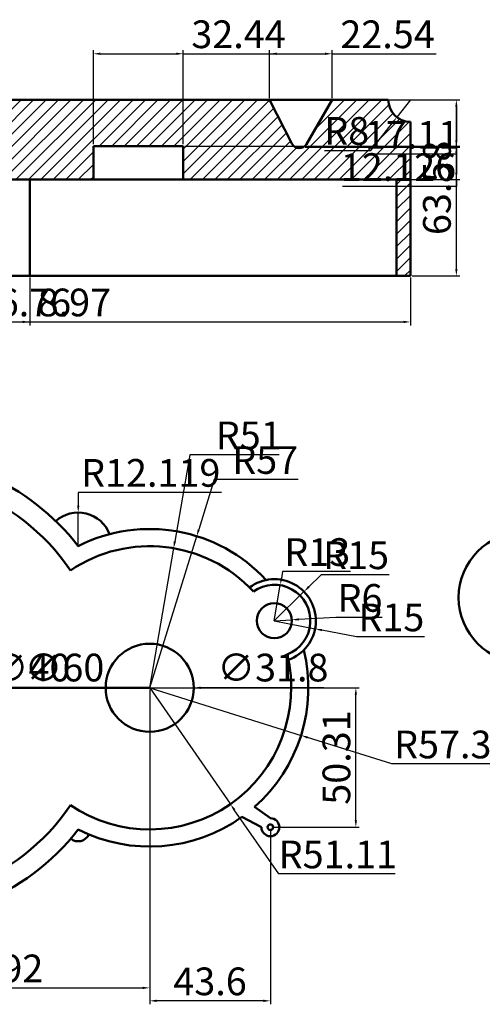
# Model space of a CAD drawing. Units: millimetres. Extents: x 828 to 2987, y 979 to 1807.
# Tile 2 of 6: x 1058 to 1225, y 1105 to 1460. Entities that reach past the tile are written whole.
import ezdxf

# ---------------------------------------------------------------- set-up
doc = ezdxf.new("R2010")
doc.units = ezdxf.units.MM
for name, color, linetype, lineweight in [('M-DIMS', 2, 'Continuous', 25), ('M-HATC', 8, 'Continuous', 18), ('M-OUTL', 7, 'Continuous', 50)]:
    doc.layers.add(name, color=color, linetype=linetype, lineweight=lineweight)
doc.styles.get("Standard").update_dxf_attribs({"font": 'arial.ttf'})
doc.dimstyles.new('ISO-25', dxfattribs={"dimtxt": 10, "dimasz": 2.5, "dimexe": 1.25, "dimexo": 0.625, "dimtad": 1, "dimtoh": 1, "dimdec": 0, "dimtxsty": 'Standard', "dimcen": 2.5, "dimadec": 0, "dimazin": 0, "dimtfac": 1, "dimtdec": 0, "dimtmove": 0, "dimatfit": 3, "dimfxl": 1, "dimarcsym": 0})

# ---------------------------------------------------------------- blocks, each defined once
blk = doc.blocks.new('*D17')
at = {"layer": 'Defpoints', "color": 0, "transparency": 16777216}
for p in [(1013.21, 1219.26), (1105.21, 1219.26), (1105.21, 1110.96)]:
    blk.add_point(p, dxfattribs=at)
at = {"layer": 'M-DIMS', "color": 0, "lineweight": -2, "transparency": 16777216}
for p, q in [((1013.21, 1218.63), (1013.21, 1109.71)), ((1105.21, 1218.63), (1105.21, 1109.71)), ((1015.71, 1110.96), (1102.71, 1110.96))]:
    blk.add_line(p, q, dxfattribs=at)
at = {"layer": 'M-DIMS', "color": 0, "transparency": 16777216}
for points in [[(1015.71, 1111.37), (1015.71, 1110.54), (1013.21, 1110.96)], [(1102.71, 1111.37), (1102.71, 1110.54), (1105.21, 1110.96)]]:
    blk.add_solid(points, dxfattribs=at)
at = {"layer": 'M-DIMS', "color": 0, "transparency": 16777216, "insert": (1059.21, 1116.69), "char_height": 10, "attachment_point": 5}
blk.add_mtext('92', dxfattribs=at)
blk = doc.blocks.new('*D20')
at = {"layer": 'Defpoints', "color": 0, "transparency": 16777216}
for p in [(1122.19, 1273.99), (1105.21, 1219.26)]:
    blk.add_point(p, dxfattribs=at)
at = {"layer": 'M-DIMS', "color": 0, "lineweight": -2, "transparency": 16777216}
for p, q in [((1128.54, 1294.46), (1122.93, 1276.38)), ((1158.89, 1294.46), (1128.54, 1294.46)), ((1105.21, 1219.26), (1122.19, 1273.99))]:
    blk.add_line(p, q, dxfattribs=at)
at = {"layer": 'M-DIMS', "color": 0, "transparency": 16777216}
blk.add_solid([(1122.54, 1276.5), (1123.33, 1276.25), (1122.19, 1273.99)], dxfattribs=at)
at = {"layer": 'M-DIMS', "color": 0, "transparency": 16777216, "insert": (1146.94, 1300.17), "char_height": 10, "attachment_point": 5}
blk.add_mtext('R57', dxfattribs=at)
blk = doc.blocks.new('*D21')
at = {"layer": 'Defpoints', "color": 0, "transparency": 16777216}
for p in [(1113.88, 1269.63), (1105.21, 1219.26)]:
    blk.add_point(p, dxfattribs=at)
at = {"layer": 'M-DIMS', "color": 0, "lineweight": -2, "transparency": 16777216}
for p, q in [((1119.67, 1303.32), (1114.3, 1272.1)), ((1151.97, 1303.32), (1119.67, 1303.32)), ((1105.21, 1219.26), (1113.88, 1269.63))]:
    blk.add_line(p, q, dxfattribs=at)
at = {"layer": 'M-DIMS', "color": 0, "transparency": 16777216}
blk.add_solid([(1113.89, 1272.17), (1114.71, 1272.03), (1113.88, 1269.63)], dxfattribs=at)
at = {"layer": 'M-DIMS', "color": 0, "transparency": 16777216, "insert": (1140.99, 1309.06), "char_height": 10, "attachment_point": 5}
blk.add_mtext('R51', dxfattribs=at)
blk = doc.blocks.new('*D22')
at = {"layer": 'Defpoints', "color": 0, "transparency": 16777216}
for p in [(1152.36, 1256.28), (1150.24, 1243.45)]:
    blk.add_point(p, dxfattribs=at)
at = {"layer": 'M-DIMS', "color": 0, "lineweight": -2, "transparency": 16777216}
for p, q in [((1153.18, 1261.21), (1152.77, 1258.74)), ((1177.7, 1261.21), (1153.18, 1261.21)), ((1150.24, 1243.45), (1152.36, 1256.28))]:
    blk.add_line(p, q, dxfattribs=at)
at = {"layer": 'M-DIMS', "color": 0, "transparency": 16777216}
blk.add_solid([(1152.36, 1258.81), (1153.18, 1258.68), (1152.36, 1256.28)], dxfattribs=at)
at = {"layer": 'M-DIMS', "color": 0, "transparency": 16777216, "insert": (1165.75, 1266.94), "char_height": 10, "attachment_point": 5}
blk.add_mtext('R13', dxfattribs=at)
blk = doc.blocks.new('*D23')
at = {"layer": 'Defpoints', "color": 0, "transparency": 16777216}
for p in [(1160.95, 1253.96), (1150.24, 1243.45)]:
    blk.add_point(p, dxfattribs=at)
at = {"layer": 'M-DIMS', "color": 0, "lineweight": -2, "transparency": 16777216}
for p, q in [((1167.16, 1260.06), (1162.73, 1255.71)), ((1191.76, 1260.06), (1167.16, 1260.06)), ((1150.24, 1243.45), (1160.95, 1253.96))]:
    blk.add_line(p, q, dxfattribs=at)
at = {"layer": 'M-DIMS', "color": 0, "transparency": 16777216}
blk.add_solid([(1162.44, 1256.01), (1163.02, 1255.41), (1160.95, 1253.96)], dxfattribs=at)
at = {"layer": 'M-DIMS', "color": 0, "transparency": 16777216, "insert": (1179.77, 1265.79), "char_height": 10, "attachment_point": 5}
blk.add_mtext('R15', dxfattribs=at)
blk = doc.blocks.new('*D24')
at = {"layer": 'Defpoints', "color": 0, "transparency": 16777216}
for p in [(1156.56, 1243.8), (1150.24, 1243.45)]:
    blk.add_point(p, dxfattribs=at)
at = {"layer": 'M-DIMS', "color": 0, "lineweight": -2, "transparency": 16777216}
for p, q in [((1150.24, 1243.45), (1156.56, 1243.8)), ((1172.5, 1244.66), (1159.06, 1243.93)), ((1189.25, 1244.66), (1172.5, 1244.66))]:
    blk.add_line(p, q, dxfattribs=at)
at = {"layer": 'M-DIMS', "color": 0, "transparency": 16777216}
blk.add_solid([(1159.04, 1244.35), (1159.08, 1243.52), (1156.56, 1243.8)], dxfattribs=at)
at = {"layer": 'M-DIMS', "color": 0, "transparency": 16777216, "insert": (1181.19, 1250.4), "char_height": 10, "attachment_point": 5}
blk.add_mtext('R6', dxfattribs=at)
blk = doc.blocks.new('*D78')
at = {"layer": 'Defpoints', "color": 0, "transparency": 16777216}
for p in [(1105.21, 1219.26), (1148.82, 1168.95), (1105.21, 1106.29)]:
    blk.add_point(p, dxfattribs=at)
at = {"layer": 'M-DIMS', "color": 0, "lineweight": -2, "transparency": 16777216}
for p, q in [((1105.21, 1218.63), (1105.21, 1105.04)), ((1148.82, 1168.33), (1148.82, 1105.04)), ((1146.32, 1106.29), (1107.71, 1106.29))]:
    blk.add_line(p, q, dxfattribs=at)
at = {"layer": 'M-DIMS', "color": 0, "transparency": 16777216}
for points in [[(1107.71, 1106.7), (1107.71, 1105.87), (1105.21, 1106.29)], [(1146.32, 1106.7), (1146.32, 1105.87), (1148.82, 1106.29)]]:
    blk.add_solid(points, dxfattribs=at)
at = {"layer": 'M-DIMS', "color": 0, "transparency": 16777216, "insert": (1127.02, 1112.02), "char_height": 10, "attachment_point": 5}
blk.add_mtext('43.6', dxfattribs=at)
blk = doc.blocks.new('*D79')
at = {"layer": 'Defpoints', "color": 0, "transparency": 16777216}
for p in [(1105.21, 1219.26), (1179.69, 1219.26), (1148.82, 1168.95)]:
    blk.add_point(p, dxfattribs=at)
at = {"layer": 'M-DIMS', "color": 0, "lineweight": -2, "transparency": 16777216}
for p, q in [((1105.84, 1219.26), (1180.94, 1219.26)), ((1179.69, 1171.45), (1179.69, 1216.76)), ((1149.44, 1168.95), (1180.94, 1168.95))]:
    blk.add_line(p, q, dxfattribs=at)
at = {"layer": 'M-DIMS', "color": 0, "transparency": 16777216}
for points in [[(1179.28, 1216.76), (1180.11, 1216.76), (1179.69, 1219.26)], [(1179.28, 1171.45), (1180.11, 1171.45), (1179.69, 1168.95)]]:
    blk.add_solid(points, dxfattribs=at)
at = {"layer": 'M-DIMS', "color": 0, "transparency": 16777216, "insert": (1173.96, 1194.1), "char_height": 10, "attachment_point": 5, "rotation": 90}
blk.add_mtext('50.31', dxfattribs=at)
blk = doc.blocks.new('*D80')
at = {"layer": 'Defpoints', "color": 0, "transparency": 16777216}
for p in [(912.63, 1367.9), (1199.4, 1367.9), (1199.4, 1351.3)]:
    blk.add_point(p, dxfattribs=at)
at = {"layer": 'M-DIMS', "color": 0, "lineweight": -2, "transparency": 16777216}
for p, q in [((912.63, 1367.28), (912.63, 1350.05)), ((1199.4, 1367.28), (1199.4, 1350.05)), ((915.13, 1351.3), (1196.9, 1351.3))]:
    blk.add_line(p, q, dxfattribs=at)
at = {"layer": 'M-DIMS', "color": 0, "transparency": 16777216}
for points in [[(915.13, 1351.72), (915.13, 1350.88), (912.63, 1351.3)], [(1196.9, 1351.72), (1196.9, 1350.88), (1199.4, 1351.3)]]:
    blk.add_solid(points, dxfattribs=at)
at = {"layer": 'M-DIMS', "color": 0, "transparency": 16777216, "insert": (1056.02, 1357.03), "char_height": 10, "attachment_point": 5}
blk.add_mtext('286.76', dxfattribs=at)
blk = doc.blocks.new('*D81')
at = {"layer": 'Defpoints', "color": 0, "transparency": 16777216}
for p in [(1191.4, 1431.48), (1216, 1431.48), (1199.4, 1367.9)]:
    blk.add_point(p, dxfattribs=at)
at = {"layer": 'M-DIMS', "color": 0, "lineweight": -2, "transparency": 16777216}
for p, q in [((1192.02, 1431.48), (1217.25, 1431.48)), ((1216, 1370.4), (1216, 1428.98)), ((1200.02, 1367.9), (1217.25, 1367.9))]:
    blk.add_line(p, q, dxfattribs=at)
at = {"layer": 'M-DIMS', "color": 0, "transparency": 16777216}
for points in [[(1215.58, 1428.98), (1216.41, 1428.98), (1216, 1431.48)], [(1215.58, 1370.4), (1216.41, 1370.4), (1216, 1367.9)]]:
    blk.add_solid(points, dxfattribs=at)
at = {"layer": 'M-DIMS', "color": 0, "transparency": 16777216, "insert": (1210.26, 1399.69), "char_height": 10, "attachment_point": 5, "rotation": 90}
blk.add_mtext('63.58', dxfattribs=at)
blk = doc.blocks.new('*D88')
at = {"layer": 'Defpoints', "color": 0, "transparency": 16777216}
for p in [(1117.32, 1448.08), (1084.88, 1414.78), (1117.32, 1414.78)]:
    blk.add_point(p, dxfattribs=at)
at = {"layer": 'M-DIMS', "color": 0, "lineweight": -2, "transparency": 16777216}
for p, q in [((1084.88, 1415.41), (1084.88, 1449.33)), ((1087.38, 1448.08), (1114.82, 1448.08)), ((1117.32, 1415.41), (1117.32, 1449.33)), ((1117.32, 1448.08), (1154.77, 1448.08))]:
    blk.add_line(p, q, dxfattribs=at)
at = {"layer": 'M-DIMS', "color": 0, "transparency": 16777216}
for points in [[(1087.38, 1448.5), (1087.38, 1447.67), (1084.88, 1448.08)], [(1114.82, 1448.5), (1114.82, 1447.67), (1117.32, 1448.08)]]:
    blk.add_solid(points, dxfattribs=at)
at = {"layer": 'M-DIMS', "color": 0, "transparency": 16777216, "insert": (1137.3, 1453.82), "char_height": 10, "attachment_point": 5}
blk.add_mtext('32.44', dxfattribs=at)
blk = doc.blocks.new('*D89')
at = {"layer": 'Defpoints', "color": 0, "transparency": 16777216}
for p in [(1117.32, 1414.78), (1117.32, 1402.66), (1216, 1402.66)]:
    blk.add_point(p, dxfattribs=at)
at = {"layer": 'M-DIMS', "color": 0, "lineweight": -2, "transparency": 16777216}
for p, q in [((1117.95, 1414.78), (1217.25, 1414.78)), ((1216, 1412.28), (1216, 1405.16)), ((1117.95, 1402.66), (1217.25, 1402.66)), ((1216, 1400.16), (1174.81, 1400.16)), ((1216, 1402.66), (1216, 1400.16))]:
    blk.add_line(p, q, dxfattribs=at)
at = {"layer": 'M-DIMS', "color": 0, "transparency": 16777216}
for points in [[(1215.58, 1412.28), (1216.41, 1412.28), (1216, 1414.78)], [(1215.58, 1405.16), (1216.41, 1405.16), (1216, 1402.66)]]:
    blk.add_solid(points, dxfattribs=at)
at = {"layer": 'M-DIMS', "color": 0, "transparency": 16777216, "insert": (1195.09, 1405.89), "char_height": 10, "attachment_point": 5}
blk.add_mtext('12.126', dxfattribs=at)
blk = doc.blocks.new('*D90')
at = {"layer": 'Defpoints', "color": 0, "transparency": 16777216}
for p in [(1148.54, 1431.48), (1160.69, 1414.37), (1216, 1414.37)]:
    blk.add_point(p, dxfattribs=at)
at = {"layer": 'M-DIMS', "color": 0, "lineweight": -2, "transparency": 16777216}
for p, q in [((1149.16, 1431.48), (1217.25, 1431.48)), ((1216, 1428.98), (1216, 1416.87)), ((1161.32, 1414.37), (1217.25, 1414.37)), ((1216, 1414.37), (1216, 1411.87)), ((1216, 1411.87), (1184.5, 1411.87))]:
    blk.add_line(p, q, dxfattribs=at)
at = {"layer": 'M-DIMS', "color": 0, "transparency": 16777216}
for points in [[(1215.58, 1428.98), (1216.41, 1428.98), (1216, 1431.48)], [(1215.58, 1416.87), (1216.41, 1416.87), (1216, 1414.37)]]:
    blk.add_solid(points, dxfattribs=at)
at = {"layer": 'M-DIMS', "color": 0, "transparency": 16777216, "insert": (1199.94, 1417.52), "char_height": 10, "attachment_point": 5}
blk.add_mtext('17.11', dxfattribs=at)
blk = doc.blocks.new('*D92')
at = {"layer": 'Defpoints', "color": 0, "transparency": 16777216}
for p in [(1052.92, 1367.9), (1061.89, 1367.9), (1061.89, 1351.3)]:
    blk.add_point(p, dxfattribs=at)
at = {"layer": 'M-DIMS', "color": 0, "lineweight": -2, "transparency": 16777216}
for p, q in [((1052.92, 1367.28), (1052.92, 1350.05)), ((1061.89, 1367.28), (1061.89, 1350.05)), ((1055.42, 1351.3), (1059.39, 1351.3)), ((1061.89, 1351.3), (1091.63, 1351.3))]:
    blk.add_line(p, q, dxfattribs=at)
at = {"layer": 'M-DIMS', "color": 0, "transparency": 16777216}
for points in [[(1055.42, 1351.72), (1055.42, 1350.88), (1052.92, 1351.3)], [(1059.39, 1351.72), (1059.39, 1350.88), (1061.89, 1351.3)]]:
    blk.add_solid(points, dxfattribs=at)
at = {"layer": 'M-DIMS', "color": 0, "transparency": 16777216, "insert": (1078.01, 1357.03), "char_height": 10, "attachment_point": 5}
blk.add_mtext('8.97', dxfattribs=at)
blk = doc.blocks.new('*D93')
at = {"layer": 'Defpoints', "color": 0, "transparency": 16777216}
for p in [(1171.08, 1448.08), (1148.54, 1431.48), (1171.08, 1431.48)]:
    blk.add_point(p, dxfattribs=at)
at = {"layer": 'M-DIMS', "color": 0, "lineweight": -2, "transparency": 16777216}
for p, q in [((1148.54, 1432.11), (1148.54, 1449.33)), ((1151.04, 1448.08), (1168.58, 1448.08)), ((1171.08, 1432.11), (1171.08, 1449.33)), ((1171.08, 1448.08), (1208.7, 1448.08))]:
    blk.add_line(p, q, dxfattribs=at)
at = {"layer": 'M-DIMS', "color": 0, "transparency": 16777216}
for points in [[(1151.04, 1448.5), (1151.04, 1447.67), (1148.54, 1448.08)], [(1168.58, 1448.5), (1168.58, 1447.67), (1171.08, 1448.08)]]:
    blk.add_solid(points, dxfattribs=at)
at = {"layer": 'M-DIMS', "color": 0, "transparency": 16777216, "insert": (1191.14, 1453.81), "char_height": 10, "attachment_point": 5}
blk.add_mtext('22.54', dxfattribs=at)
blk = doc.blocks.new('*D126')
at = {"layer": 'Defpoints', "color": 0, "transparency": 16777216}
for p in [(983.21, 1219.26), (1043.21, 1219.26)]:
    blk.add_point(p, dxfattribs=at)
at = {"layer": 'M-DIMS', "color": 0, "lineweight": -2, "transparency": 16777216}
for p, q in [((980.71, 1219.26), (978.21, 1219.26)), ((983.21, 1219.26), (1043.21, 1219.26)), ((1061.21, 1219.26), (1045.71, 1219.26)), ((1087.01, 1219.26), (1061.21, 1219.26))]:
    blk.add_line(p, q, dxfattribs=at)
at = {"layer": 'M-DIMS', "color": 0, "transparency": 16777216}
for points in [[(980.71, 1219.68), (980.71, 1218.84), (983.21, 1219.26)], [(1045.71, 1219.68), (1045.71, 1218.84), (1043.21, 1219.26)]]:
    blk.add_solid(points, dxfattribs=at)
at = {"layer": 'M-DIMS', "color": 0, "transparency": 16777216, "insert": (1074.43, 1225.27), "char_height": 10, "attachment_point": 5}
blk.add_mtext('∅60', dxfattribs=at)
blk = doc.blocks.new('*D127')
at = {"layer": 'Defpoints', "color": 0, "transparency": 16777216}
for p in [(993.21, 1219.26), (1033.21, 1219.26)]:
    blk.add_point(p, dxfattribs=at)
at = {"layer": 'M-DIMS', "color": 0, "lineweight": -2, "transparency": 16777216}
for p, q in [((990.71, 1219.26), (988.21, 1219.26)), ((993.21, 1219.26), (1033.21, 1219.26)), ((1048.99, 1219.26), (1035.71, 1219.26)), ((1074.78, 1219.26), (1048.99, 1219.26))]:
    blk.add_line(p, q, dxfattribs=at)
at = {"layer": 'M-DIMS', "color": 0, "transparency": 16777216}
for points in [[(990.71, 1219.68), (990.71, 1218.84), (993.21, 1219.26)], [(1035.71, 1219.68), (1035.71, 1218.84), (1033.21, 1219.26)]]:
    blk.add_solid(points, dxfattribs=at)
at = {"layer": 'M-DIMS', "color": 0, "transparency": 16777216, "insert": (1062.2, 1225.27), "char_height": 10, "attachment_point": 5}
blk.add_mtext('∅40', dxfattribs=at)
blk = doc.blocks.new('*D128')
at = {"layer": 'Defpoints', "color": 0, "transparency": 16777216}
for p in [(1105.21, 1219.26), (1159.88, 1202.09)]:
    blk.add_point(p, dxfattribs=at)
at = {"layer": 'M-DIMS', "color": 0, "lineweight": -2, "transparency": 16777216}
for p, q in [((1105.21, 1219.26), (1159.88, 1202.09)), ((1192.68, 1191.78), (1162.27, 1201.34)), ((1228.86, 1191.78), (1192.68, 1191.78))]:
    blk.add_line(p, q, dxfattribs=at)
at = {"layer": 'M-DIMS', "color": 0, "transparency": 16777216}
blk.add_solid([(1162.39, 1201.73), (1162.14, 1200.94), (1159.88, 1202.09)], dxfattribs=at)
at = {"layer": 'M-DIMS', "color": 0, "transparency": 16777216, "insert": (1211.08, 1197.51), "char_height": 10, "attachment_point": 5}
blk.add_mtext('R57.3', dxfattribs=at)
blk = doc.blocks.new('*D129')
at = {"layer": 'Defpoints', "color": 0, "transparency": 16777216}
for p in [(1105.21, 1219.26), (1134.37, 1177.28)]:
    blk.add_point(p, dxfattribs=at)
at = {"layer": 'M-DIMS', "color": 0, "lineweight": -2, "transparency": 16777216}
for p, q in [((1105.21, 1219.26), (1134.37, 1177.28)), ((1151.86, 1152.08), (1135.79, 1175.22)), ((1193.87, 1152.08), (1151.86, 1152.08))]:
    blk.add_line(p, q, dxfattribs=at)
at = {"layer": 'M-DIMS', "color": 0, "transparency": 16777216}
blk.add_solid([(1136.13, 1175.46), (1135.45, 1174.98), (1134.37, 1177.28)], dxfattribs=at)
at = {"layer": 'M-DIMS', "color": 0, "transparency": 16777216, "insert": (1173.18, 1157.82), "char_height": 10, "attachment_point": 5}
blk.add_mtext('R51.11', dxfattribs=at)
blk = doc.blocks.new('*D130')
at = {"layer": 'Defpoints', "color": 0, "transparency": 16777216}
for p in [(1089.32, 1219.26), (1121.11, 1219.26)]:
    blk.add_point(p, dxfattribs=at)
at = {"layer": 'M-DIMS', "color": 0, "lineweight": -2, "transparency": 16777216}
for p, q in [((1086.82, 1219.26), (1084.32, 1219.26)), ((1089.32, 1219.26), (1121.11, 1219.26)), ((1130.65, 1219.26), (1123.61, 1219.26)), ((1168.15, 1219.26), (1130.65, 1219.26))]:
    blk.add_line(p, q, dxfattribs=at)
at = {"layer": 'M-DIMS', "color": 0, "transparency": 16777216}
for points in [[(1086.82, 1219.68), (1086.82, 1218.84), (1089.32, 1219.26)], [(1123.61, 1219.68), (1123.61, 1218.84), (1121.11, 1219.26)]]:
    blk.add_solid(points, dxfattribs=at)
at = {"layer": 'M-DIMS', "color": 0, "transparency": 16777216, "insert": (1149.72, 1225.27), "char_height": 10, "attachment_point": 5}
blk.add_mtext('∅31.8', dxfattribs=at)
blk = doc.blocks.new('*D131')
at = {"layer": 'Defpoints', "color": 0, "transparency": 16777216}
for p in [(1150.24, 1243.45), (1164.96, 1240.57)]:
    blk.add_point(p, dxfattribs=at)
at = {"layer": 'M-DIMS', "color": 0, "lineweight": -2, "transparency": 16777216}
for p, q in [((1150.24, 1243.45), (1164.96, 1240.57)), ((1179.89, 1237.64), (1167.41, 1240.09)), ((1204.48, 1237.64), (1179.89, 1237.64))]:
    blk.add_line(p, q, dxfattribs=at)
at = {"layer": 'M-DIMS', "color": 0, "transparency": 16777216}
blk.add_solid([(1167.49, 1240.49), (1167.33, 1239.68), (1164.96, 1240.57)], dxfattribs=at)
at = {"layer": 'M-DIMS', "color": 0, "transparency": 16777216, "insert": (1192.5, 1243.37), "char_height": 10, "attachment_point": 5}
blk.add_mtext('R15', dxfattribs=at)
blk = doc.blocks.new('*D133')
at = {"layer": 'Defpoints', "color": 0, "transparency": 16777216}
for p in [(1079.4, 1282.53), (1079.38, 1270.41)]:
    blk.add_point(p, dxfattribs=at)
at = {"layer": 'M-DIMS', "color": 0, "lineweight": -2, "transparency": 16777216}
for p, q in [((1079.41, 1289.8), (1079.4, 1285.03)), ((1131.14, 1289.8), (1079.41, 1289.8)), ((1079.38, 1270.41), (1079.4, 1282.53))]:
    blk.add_line(p, q, dxfattribs=at)
at = {"layer": 'M-DIMS', "color": 0, "transparency": 16777216}
blk.add_solid([(1078.99, 1285.03), (1079.82, 1285.02), (1079.4, 1282.53)], dxfattribs=at)
at = {"layer": 'M-DIMS', "color": 0, "transparency": 16777216, "insert": (1105.59, 1295.53), "char_height": 10, "attachment_point": 5}
blk.add_mtext('R12.119', dxfattribs=at)
blk = doc.blocks.new('*D134')
at = {"layer": 'Defpoints', "color": 0, "transparency": 16777216}
for p in [(1199.4, 1431.48), (1194.47, 1425.18)]:
    blk.add_point(p, dxfattribs=at)
at = {"layer": 'M-DIMS', "color": 0, "lineweight": -2, "transparency": 16777216}
for p, q in [((1199.4, 1431.48), (1194.47, 1425.18)), ((1185.09, 1413.2), (1192.93, 1423.21)), ((1168.32, 1413.2), (1185.09, 1413.2))]:
    blk.add_line(p, q, dxfattribs=at)
at = {"layer": 'M-DIMS', "color": 0, "transparency": 16777216}
blk.add_solid([(1192.6, 1423.47), (1193.26, 1422.96), (1194.47, 1425.18)], dxfattribs=at)
at = {"layer": 'M-DIMS', "color": 0, "transparency": 16777216, "insert": (1176.4, 1418.93), "char_height": 10, "attachment_point": 5}
blk.add_mtext('R8', dxfattribs=at)

msp = doc.modelspace()

# ---------------------------------------------------------------- hatches: boundary and pattern name
at = {"layer": 'M-HATC'}
h = msp.add_hatch(dxfattribs=at)
h.set_pattern_fill('ANSI31', color=256)
h.paths.add_polyline_path([(962.2684, 1413.4084), (996.3583, 1413.4084), (996.3583, 1402.6561), (1084.8819, 1402.6561), (1084.8819, 1414.7818), (1117.3222, 1414.7818), (1117.3222, 1402.6561), (1194.3976, 1402.6561), (1194.3976, 1367.9009), (1199.3976, 1367.9009), (1199.3976, 1423.4818, -0.41421356), (1191.3976, 1431.4818), (1171.0768, 1431.4818), (1161.8287, 1415.4895, -0.59566696), (1156.5548, 1415.6369), (1148.5383, 1431.4818), (973.775, 1431.4818), (937.4085, 1410.469), (912.4339, 1409.5934), (912.6342, 1402.6561), (962.2684, 1402.6561)])

# ---------------------------------------------------------------- linework, layer by layer
at = {"layer": 'M-OUTL'}
for p, q in [((1191.3976, 1431.4818), (973.775, 1431.4818)), ((1148.5383, 1431.4818), (1156.5548, 1415.6369)), ((1161.8287, 1415.4895), (1171.0768, 1431.4818)), ((1199.3976, 1367.9009), (1199.3976, 1423.4818)), ((1084.8819, 1402.6561), (1084.8819, 1414.7818)), ((1084.8819, 1414.7818), (1117.3222, 1414.7818)), ((1117.3222, 1414.7818), (1117.3222, 1402.6561)), ((1194.3976, 1402.6561), (912.6342, 1402.6561)), ((1061.8863, 1402.6561), (1061.8863, 1367.9009)), ((1194.3976, 1367.9009), (1194.3976, 1402.6561)), ((912.6342, 1367.9009), (1194.3976, 1367.9009)), ((1194.3976, 1367.9009), (1199.3976, 1367.9009)), ((1013.2149, 1219.2594), (1105.2149, 1219.2594)), ((1148.8153, 1172.1931), (1143.0902, 1176.2584)), ((1145.5726, 1168.9504), (1138.5497, 1172.6502))]:
    msp.add_line(p, q, dxfattribs=at)
for centre, radius in [((1240.2869, 1251.8522), 23.5), ((1150.2395, 1243.4522), 6.3327), ((1105.2149, 1219.2594), 15.8988), ((1148.8153, 1168.9504), 1.0224)]:
    msp.add_circle(centre, radius, dxfattribs=at)
for centre, radius, start, end in [((1199.3976, 1431.4818), 8, 180, 270), ((1159.2317, 1416.9913), 3, 206.836506, 329.959944), ((1013.2149, 1219.2594), 83.6262, 37.706236, 153.567782), ((1013.2149, 1219.2594), 76.1927, 33.749512, 326.250488), ((1079.3763, 1270.4063), 12.1188, 20.732215, 131.86141), ((1105.2149, 1219.2594), 57.303, 42.753797, 116.802176), ((1105.2149, 1219.2594), 51.1127, 42.862262, 124.08907), ((1150.2395, 1243.4522), 15, 289.812357, 126.687829), ((1150.2395, 1243.4522), 13, 290.944009, 125.556177), ((1105.2149, 1219.2594), 51.1127, 235.91093, 13.637924), ((1105.2149, 1219.2594), 57.303, 311.373628, 13.746389), ((1105.2149, 1219.2594), 57.303, 243.197824, 305.572215), ((1148.8153, 1168.9504), 3.2427, 180, 90), ((1013.2149, 1219.2594), 83.6262, 260.664363, 322.293764), ((1079.3763, 1168.1126), 4.2506, 230.837462, 335.323363)]:
    msp.add_arc(centre, radius, start, end, dxfattribs=at)

# ---------------------------------------------------------------- dimensions: what is measured, and where the dimension line sits
at = {"layer": 'M-DIMS'}
for base, p1, p2, override, picture, middle in [((1117.3222, 1448.0818), (1084.8819, 1414.7818), (1117.3222, 1414.7818), {"dimdec": 2, "dimlfac": 1, "dimrnd": 0, "dimzin": 0, "dimdsep": 46, "dimlunit": 2}, '*D88', (1137.2958, 1453.816)), ((1171.0768, 1448.0818), (1148.5383, 1431.4818), (1171.0768, 1431.4818), {"dimdec": 2, "dimlfac": 1, "dimrnd": 0, "dimzin": 0, "dimdsep": 46, "dimlunit": 2}, '*D93', (1191.1391, 1453.8126)), ((1199.3976, 1351.3009), (912.6342, 1367.9009), (1199.3976, 1367.9009), {"dimdec": 2, "dimlfac": 1, "dimrnd": 0, "dimzin": 0, "dimdsep": 46, "dimlunit": 2}, '*D80', (1056.0159, 1357.0316)), ((1061.8863, 1351.3009), (1052.9164, 1367.9009), (1061.8863, 1367.9009), {"dimdec": 2, "dimlfac": 1, "dimrnd": 0, "dimzin": 0, "dimdsep": 46, "dimlunit": 2}, '*D92', (1078.0058, 1357.0316)), ((1105.2149, 1110.9564), (1013.2149, 1219.2594), (1105.2149, 1219.2594), {"dimclrd": 0, "dimclre": 0, "dimclrt": 0}, '*D17', (1059.2149, 1116.6871)), ((1105.2149, 1106.2871), (1148.8153, 1168.9504), (1105.2149, 1219.2594), {"dimdec": 1, "dimlfac": 1, "dimrnd": 0, "dimzin": 0, "dimdsep": 46, "dimlunit": 2}, '*D78', (1127.0151, 1112.0212))]:
    dim = msp.add_linear_dim(base=base, p1=p1, p2=p2, dimstyle='ISO-25', override=override, dxfattribs=at)
    dim.commit()
    dim.dimension.update_dxf_attribs({"geometry": picture, "text_midpoint": middle})
for base, p1, p2, override, picture, middle in [((1215.9976, 1414.372), (1148.5383, 1431.4818), (1160.6943, 1414.372), {"dimdec": 2, "dimlfac": 1, "dimrnd": 0, "dimzin": 0, "dimdsep": 46, "dimlunit": 2}, '*D90', (1199.936, 1417.5174)), ((1215.9976, 1431.4818), (1199.3976, 1367.9009), (1191.3976, 1431.4818), {"dimdec": 2, "dimlfac": 1, "dimrnd": 0, "dimzin": 0, "dimdsep": 46, "dimlunit": 2}, '*D81', (1210.2635, 1399.6914)), ((1215.9976, 1402.6561), (1117.3222, 1414.7818), (1117.3222, 1402.6561), {"dimdec": 3, "dimlfac": 1, "dimrnd": 0, "dimzin": 0, "dimdsep": 46, "dimlunit": 2}, '*D89', (1195.0895, 1405.8868)), ((1179.692, 1219.2594), (1148.8153, 1168.9504), (1105.2149, 1219.2594), {"dimdec": 2, "dimlfac": 1, "dimrnd": 0, "dimzin": 0, "dimdsep": 46, "dimlunit": 2}, '*D79', (1173.9579, 1194.1049))]:
    dim = msp.add_linear_dim(base=base, p1=p1, p2=p2, angle=90, dimstyle='ISO-25', override=override, dxfattribs=at)
    dim.commit()
    dim.dimension.update_dxf_attribs({"geometry": picture, "text_midpoint": middle})
for center, mpoint, override, picture, middle in [((1199.3976, 1431.4818), (1194.4681, 1425.181), {"dimdec": 0, "dimlfac": 1, "dimrnd": 0, "dimzin": 0, "dimdsep": 46, "dimlunit": 2}, '*D134', (1176.397, 1418.9313)), ((1150.2395, 1243.4522), (1152.3647, 1256.2773), {"dimclrd": 0, "dimclre": 0, "dimclrt": 0}, '*D22', (1165.7546, 1266.9442)), ((1150.2395, 1243.4522), (1164.9594, 1240.5668), {"dimdec": 0, "dimlfac": 1, "dimrnd": 0, "dimzin": 0, "dimdsep": 46, "dimlunit": 2}, '*D131', (1192.4968, 1243.3714))]:
    dim = msp.add_radius_dim(center=center, mpoint=mpoint, dimstyle='ISO-25', override=override, dxfattribs=at)
    dim.commit()
    dim.dimension.update_dxf_attribs({"geometry": picture, "text_midpoint": middle})
for center, mpoint, override, picture, middle in [((1105.2149, 1219.2594), (1113.8784, 1269.6326), {"dimclrd": 0, "dimclre": 0, "dimclrt": 0}, '*D21', (1140.9903, 1303.3244)), ((1105.2149, 1219.2594), (1122.1925, 1273.9896), {"dimclrd": 0, "dimclre": 0, "dimclrt": 0}, '*D20', (1146.941, 1294.4619)), ((1079.3763, 1270.4063), (1079.4, 1282.525), {"dimdec": 3, "dimlfac": 1, "dimrnd": 0, "dimzin": 0, "dimdsep": 46, "dimlunit": 2}, '*D133', (1105.5918, 1289.7963)), ((1150.2395, 1243.4522), (1160.9461, 1253.9578), {"dimclrd": 0, "dimclre": 0, "dimclrt": 0}, '*D23', (1179.7724, 1260.0575)), ((1150.2395, 1243.4522), (1156.5628, 1243.7965), {"dimclrd": 0, "dimclre": 0, "dimclrt": 0}, '*D24', (1172.5034, 1244.6644)), ((1105.2149, 1219.2594), (1159.8837, 1202.0851), {"dimdec": 1, "dimlfac": 1, "dimrnd": 0, "dimzin": 0, "dimdsep": 46, "dimlunit": 2}, '*D128', (1211.0828, 1191.7805)), ((1105.2149, 1219.2594), (1134.3668, 1177.2752), {"dimdec": 2, "dimlfac": 1, "dimrnd": 0, "dimzin": 0, "dimdsep": 46, "dimlunit": 2}, '*D129', (1173.1754, 1152.0847))]:
    dim = msp.add_radius_dim(center=center, mpoint=mpoint, dimstyle='ISO-25', override=override, dxfattribs=at)
    dim.commit()
    dim.dimension.update_dxf_attribs({"geometry": picture, "text_midpoint": middle, "dimtype": 164})
for p1, p2, override, picture, middle in [((983.2149, 1219.2599), (1043.2149, 1219.259), {"dimdec": 0, "dimlfac": 1, "dimrnd": 0, "dimzin": 0, "dimdsep": 46, "dimlunit": 2}, '*D126', (1061.2149, 1219.2587)), ((1089.316, 1219.2589), (1121.1137, 1219.26), {"dimdec": 1, "dimlfac": 1, "dimrnd": 0, "dimzin": 0, "dimdsep": 46, "dimlunit": 2}, '*D130', (1130.653, 1219.2603))]:
    dim = msp.add_diameter_dim_2p(p1=p1, p2=p2, dimstyle='ISO-25', override=override, dxfattribs=at)
    dim.commit()
    dim.dimension.update_dxf_attribs({"geometry": picture, "text_midpoint": middle, "dimtype": 163})
dim = msp.add_diameter_dim_2p(p1=(993.2149, 1219.2599), p2=(1033.2149, 1219.259), dimstyle='ISO-25', override={"dimdec": 0, "dimlfac": 1, "dimrnd": 0, "dimzin": 0, "dimdsep": 46, "dimlunit": 2}, dxfattribs=at)
dim.commit()
dim.dimension.update_dxf_attribs({"geometry": '*D127', "text_midpoint": (1048.9857, 1219.2587)})

doc.saveas('drawing.dxf')
